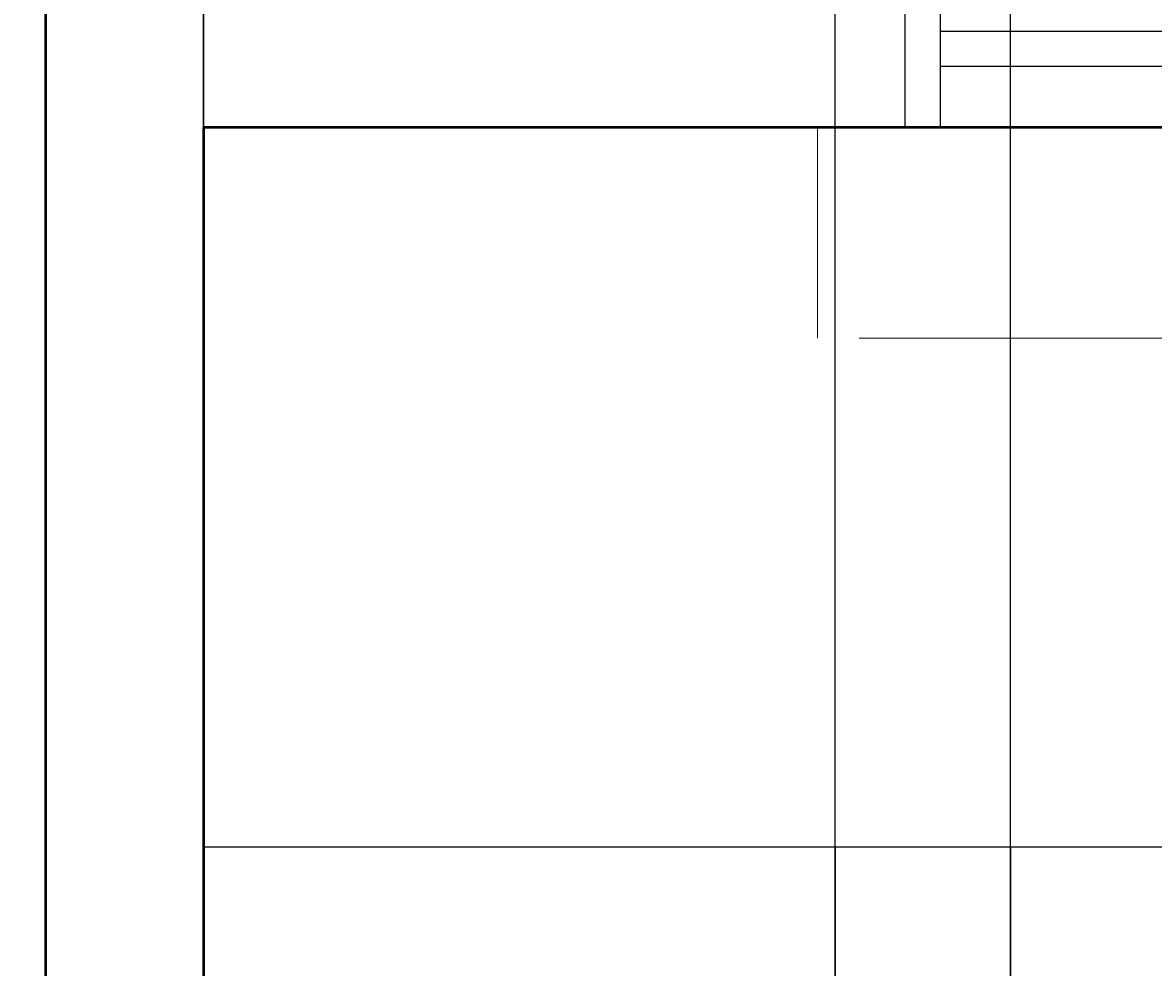
# Model space of a CAD drawing. Units: inches. Extents: x 37 to 824, y -700 to 234.
# Tile 25 of 77: x 160 to 224, y -323 to -269. Entities that reach past the tile are written whole.
import ezdxf

# ---------------------------------------------------------------- set-up
doc = ezdxf.new("R2010")
doc.units = ezdxf.units.IN
doc.header["$MEASUREMENT"] = 0
doc.linetypes.add('DASHED', pattern=[19.05, 12.7, -6.35])
for name, color, linetype, lineweight in [('A-ANNO-DIMS', 2, 'Continuous', 18), ('A-FLOR-STRS', 1, 'Continuous', 25), ('A-FLOR-STRS-OVHD', 1, 'DASHED', 18), ('A-GLAZ', 4, 'Continuous', 25), ('A-ROOF-OVHD', 1, 'DASHED', 18), ('A-WALL', 2, 'Continuous', 50)]:
    doc.layers.add(name, color=color, linetype=linetype, lineweight=lineweight)
doc.styles.get("Standard").update_dxf_attribs({"font": 'arial.ttf'})
doc.dimstyles.get("Standard").update_dxf_attribs({"dimtxt": 0.18, "dimasz": 0.18, "dimexe": 0.18, "dimexo": 0.0625, "dimgap": 0.09, "dimtad": 0, "dimtih": 1, "dimtoh": 1, "dimdec": 1, "dimzin": 0, "dimdsep": 46, "dimlunit": 4, "dimtxsty": 'Standard', "dimcen": 0.09, "dimadec": 0, "dimazin": 0, "dimtfac": 1, "dimtdec": 1, "dimtofl": 0, "dimtmove": 0, "dimatfit": 3, "dimfxl": 1, "dimtolj": 1, "dimtzin": 0, "dimarcsym": 0})

# ---------------------------------------------------------------- blocks, each defined once
blk = doc.blocks.new('WIN-900')
for p, q in [((0, 9), (0, 0)), ((2, 9), (2, 0)), ((20, 9), (20, 0)), ((38, 9), (38, 0)), ((40, 9), (40, 0)), ((38, 5.5), (2, 5.5)), ((38, 3.5), (2, 3.5))]:
    blk.add_line(p, q)
blk = doc.blocks.new('*D59')
at = {"layer": 'A-ANNO-DIMS', "color": 0, "lineweight": -2, "ltscale": 0.5, "transparency": 16777216}
for p, q in [((161.015, -236.91), (78.159, -236.91)), ((78.339, -237.09), (78.339, -301.228)), ((78.339, -365.73), (78.339, -301.591)), ((161.015, -365.91), (78.159, -365.91))]:
    blk.add_line(p, q, dxfattribs=at)
at = {"layer": 'A-ANNO-DIMS', "color": 0, "ltscale": 0.5, "transparency": 16777216}
for points in [[(78.309, -237.09), (78.369, -237.09), (78.339, -236.91)], [(78.309, -365.73), (78.369, -365.73), (78.339, -365.91)]]:
    blk.add_solid(points, dxfattribs=at)
at = {"layer": 'Defpoints', "color": 0, "ltscale": 0.5, "transparency": 16777216}
for p in [(161.077, -236.91), (78.339, -365.91), (161.077, -365.91)]:
    blk.add_point(p, dxfattribs=at)
at = {"layer": 'A-ANNO-DIMS', "color": 0, "ltscale": 0.5, "transparency": 16777216, "insert": (78.339, -301.41), "char_height": 0.18, "attachment_point": 5}
blk.add_mtext('\\A1;10\'-9"', dxfattribs=at)
blk = doc.blocks.new('*D80')
at = {"layer": 'A-ANNO-DIMS', "color": 0, "lineweight": -2, "ltscale": 0.5, "transparency": 16777216}
for p, q in [((170.077, -167.972), (170.077, -400.406)), ((250.19, -167.972), (250.19, -400.406)), ((170.257, -400.226), (209.804, -400.226)), ((250.01, -400.226), (210.463, -400.226))]:
    blk.add_line(p, q, dxfattribs=at)
at = {"layer": 'A-ANNO-DIMS', "color": 0, "ltscale": 0.5, "transparency": 16777216}
for points in [[(170.257, -400.196), (170.257, -400.256), (170.077, -400.226)], [(250.01, -400.196), (250.01, -400.256), (250.19, -400.226)]]:
    blk.add_solid(points, dxfattribs=at)
at = {"layer": 'Defpoints', "color": 0, "ltscale": 0.5, "transparency": 16777216}
for p in [(170.077, -167.91), (250.19, -167.91), (250.19, -400.226)]:
    blk.add_point(p, dxfattribs=at)
at = {"layer": 'A-ANNO-DIMS', "color": 0, "ltscale": 0.5, "transparency": 16777216, "insert": (210.133, -400.226), "char_height": 0.18, "attachment_point": 5}
blk.add_mtext('\\A1;6\'-8"', dxfattribs=at)
blk = doc.blocks.new('*D85')
at = {"layer": 'A-ANNO-DIMS', "color": 0, "lineweight": -2, "ltscale": 0.5, "transparency": 16777216}
for p, q in [((170.077, -356.847), (170.077, 234.17)), ((170.257, 233.99), (187.748, 233.99)), ((205.897, 233.99), (188.406, 233.99)), ((206.077, -356.847), (206.077, 234.17))]:
    blk.add_line(p, q, dxfattribs=at)
at = {"layer": 'A-ANNO-DIMS', "color": 0, "ltscale": 0.5, "transparency": 16777216}
for points in [[(170.257, 234.02), (170.257, 233.96), (170.077, 233.99)], [(205.897, 234.02), (205.897, 233.96), (206.077, 233.99)]]:
    blk.add_solid(points, dxfattribs=at)
at = {"layer": 'Defpoints', "color": 0, "ltscale": 0.5, "transparency": 16777216}
for p in [(206.077, 233.99), (170.077, -356.91), (206.077, -356.91)]:
    blk.add_point(p, dxfattribs=at)
at = {"layer": 'A-ANNO-DIMS', "color": 0, "ltscale": 0.5, "transparency": 16777216, "insert": (188.077, 233.99), "char_height": 0.18, "attachment_point": 5}
blk.add_mtext('\\A1;3\'-0"', dxfattribs=at)
blk = doc.blocks.new('*D86')
at = {"layer": 'A-ANNO-DIMS', "color": 0, "lineweight": -2, "ltscale": 0.5, "transparency": 16777216}
for p, q in [((206.077, -356.847), (206.077, 234.17)), ((206.257, 233.99), (210.678, 233.99)), ((215.897, 233.99), (211.476, 233.99)), ((216.077, -356.847), (216.077, 234.17))]:
    blk.add_line(p, q, dxfattribs=at)
at = {"layer": 'A-ANNO-DIMS', "color": 0, "ltscale": 0.5, "transparency": 16777216}
for points in [[(206.257, 234.02), (206.257, 233.96), (206.077, 233.99)], [(215.897, 234.02), (215.897, 233.96), (216.077, 233.99)]]:
    blk.add_solid(points, dxfattribs=at)
at = {"layer": 'Defpoints', "color": 0, "ltscale": 0.5, "transparency": 16777216}
for p in [(216.077, 233.99), (206.077, -356.91), (216.077, -356.91)]:
    blk.add_point(p, dxfattribs=at)
at = {"layer": 'A-ANNO-DIMS', "color": 0, "ltscale": 0.5, "transparency": 16777216, "insert": (211.077, 233.99), "char_height": 0.18, "attachment_point": 5}
blk.add_mtext('\\A1;0\'-10"', dxfattribs=at)
blk = doc.blocks.new('*D87')
at = {"layer": 'A-ANNO-DIMS', "color": 0, "lineweight": -2, "ltscale": 0.5, "transparency": 16777216}
for p, q in [((216.077, -356.847), (216.077, 234.17)), ((216.257, 233.99), (255.747, 233.99)), ((295.897, 233.99), (256.407, 233.99)), ((296.077, -356.847), (296.077, 234.17))]:
    blk.add_line(p, q, dxfattribs=at)
at = {"layer": 'A-ANNO-DIMS', "color": 0, "ltscale": 0.5, "transparency": 16777216}
for points in [[(216.257, 234.02), (216.257, 233.96), (216.077, 233.99)], [(295.897, 234.02), (295.897, 233.96), (296.077, 233.99)]]:
    blk.add_solid(points, dxfattribs=at)
at = {"layer": 'Defpoints', "color": 0, "ltscale": 0.5, "transparency": 16777216}
for p in [(296.077, 233.99), (216.077, -356.91), (296.077, -356.91)]:
    blk.add_point(p, dxfattribs=at)
at = {"layer": 'A-ANNO-DIMS', "color": 0, "ltscale": 0.5, "transparency": 16777216, "insert": (256.077, 233.99), "char_height": 0.18, "attachment_point": 5}
blk.add_mtext('\\A1;6\'-8"', dxfattribs=at)

msp = doc.modelspace()

# ---------------------------------------------------------------- linework, layer by layer
at = {"layer": 'A-FLOR-STRS'}
for p, q in [((170.077, -315.91), (296.077, -315.91)), ((206.077, -315.91), (206.077, -356.91)), ((216.077, -315.91), (216.077, -356.91))]:
    msp.add_line(p, q, dxfattribs=at)
at = {"layer": 'A-FLOR-STRS-OVHD'}
for p, q in [((206.077, -315.91), (206.077, -274.91)), ((216.077, -315.91), (216.077, -274.91))]:
    msp.add_line(p, q, dxfattribs=at)
at = {"layer": 'A-ROOF-OVHD', "ltscale": 1.5}
for p, q in [((210.077, -274.91), (205.077, -274.91)), ((205.077, -274.91), (205.077, -286.91)), ((255.077, -286.91), (205.077, -286.91))]:
    msp.add_line(p, q, dxfattribs=at)
at = {"layer": 'A-WALL'}
for p, q in [((161.077, 75.09), (161.077, -365.91)), ((299.077, -274.91), (170.077, -274.91)), ((170.077, -274.91), (170.077, -356.91))]:
    msp.add_line(p, q, dxfattribs=at)

# ---------------------------------------------------------------- block references
at = {"layer": 'A-GLAZ', "rotation": 180}
msp.add_blockref('WIN-900', (250.077, -265.909), dxfattribs=at)

# ---------------------------------------------------------------- dimensions: what is measured, and where the dimension line sits
at = {"layer": 'A-ANNO-DIMS', "ltscale": 0.5}
for base, p1, p2, picture, middle in [((206.077, 233.99), (170.077, -356.91), (206.077, -356.91), '*D85', (188.077, 233.99)), ((216.077, 233.99), (206.077, -356.91), (216.077, -356.91), '*D86', (211.077, 233.99)), ((296.077, 233.99), (216.077, -356.91), (296.077, -356.91), '*D87', (256.077, 233.99)), ((250.19, -400.226), (170.077, -167.91), (250.19, -167.91), '*D80', (210.133, -400.226))]:
    dim = msp.add_linear_dim(base=base, p1=p1, p2=p2, dimstyle='Standard', override={"dimdec": 1, "dimlfac": 1, "dimrnd": 0, "dimzin": 1, "dimdsep": 46, "dimlunit": 4, "dimfrac": 2}, dxfattribs=at)
    dim.commit()
    dim.dimension.update_dxf_attribs({"geometry": picture, "text_midpoint": middle})
dim = msp.add_linear_dim(base=(78.339, -365.91), p1=(161.077, -236.91), p2=(161.077, -365.91), angle=90, dimstyle='Standard', override={"dimdec": 1, "dimlfac": 1, "dimrnd": 0, "dimzin": 1, "dimdsep": 46, "dimlunit": 4, "dimfrac": 2}, dxfattribs=at)
dim.commit()
dim.dimension.update_dxf_attribs({"geometry": '*D59', "text_midpoint": (78.339, -301.41)})

doc.saveas('drawing.dxf')
